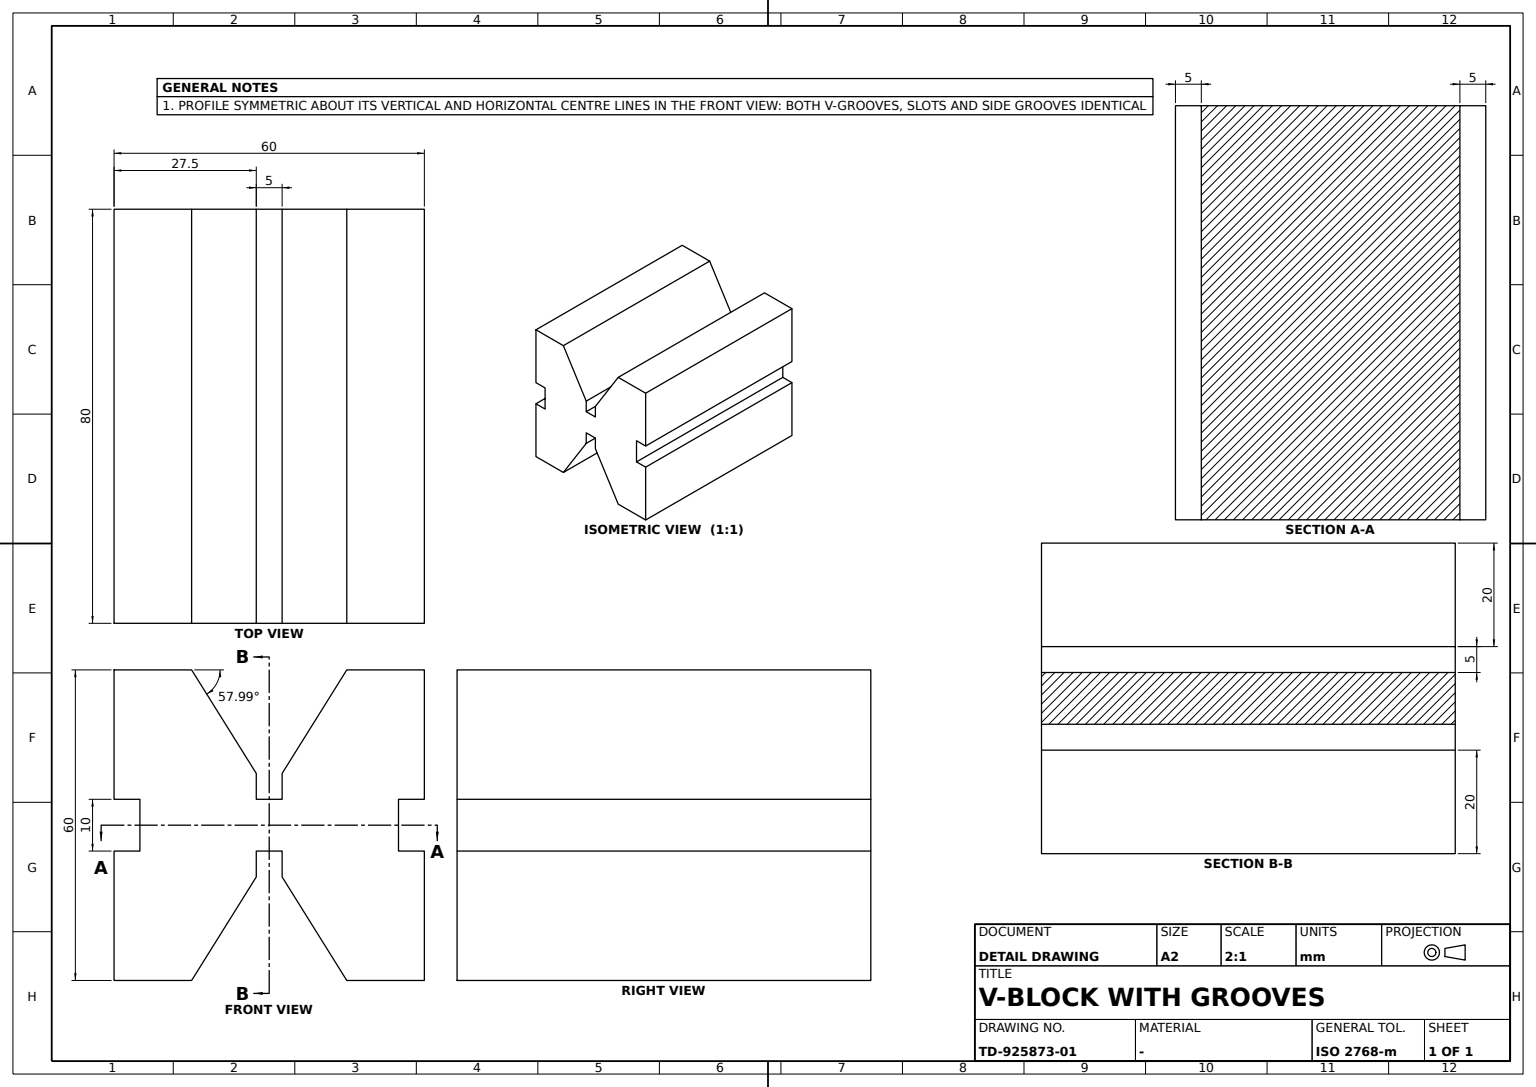
CATIA V5 part; units mm, degrees
sketch "Sketch1" plane through (0, 0, 0) normal (1, 0, 0) x (0, 1, 0)
  point P0 (15, 30)
  line L0 (15, 30) -> (30, 30)
  line L1 (30, 30) -> (30, 5)
  line L2 (30, 5) -> (25, 5)
  line L3 (25, 5) -> (25, -5)
  line L4 (25, -5) -> (30, -5)
  point P1 (30, -5)
  line L5 (30, -5) -> (30, -30)
  line L6 (30, -30) -> (15, -30)
  point P2 (15, -30)
  point P3 (0, 5)
  line L7 (0, 5) -> (2.5, 5)
  point P4 (2.5, 5)
  line L8 (2.5, 5) -> (2.5, 10)
  point P5 (2.5, 10)
  line L9 (2.5, 10) -> (15, 30)
  line L10 (0, 5) -> (0, -5)
  point P6 (0, -5)
  point P7 (15, -30)
  point P8 (2.5, -10)
  line L11 (2.5, -10) -> (15, -30)
  point P9 (2.5, -5)
  line L12 (2.5, -5) -> (2.5, -10)
  point P10 (0, -5)
  line L13 (0, -5) -> (2.5, -5)
  dimension "length L0" = 15
  dimension "length L4" = 5
  dimension "distance L2 L4" = 10
  dimension "distance L0 L6" = 60
  dimension "distance L10 P2" = 15
  dimension "length L7" = 2.5
  dimension "length L12" = 5
  dimension "length L10" = 10
  constraint horizontal L0 x-axis
  constraint horizontal L2 x-axis
  constraint horizontal L4 x-axis
  constraint horizontal L6 x-axis
  constraint horizontal L7 x-axis
  constraint vertical L1 y-axis
  constraint vertical L3 y-axis
  constraint vertical L5 y-axis
  constraint vertical L8 y-axis
  constraint vertical L10 y-axis
  constraint coincidence P1 L1
  constraint coincidence P3 y-axis
  constraint coincidence P6 P10
  constraint coincidence P2 P7
  constraint equal size L1 L5
  constraint equal size L0 L6
  constraint equal size L2 L4
  constraint symmetry L2 L4 x-axis
  constraint symmetry P0 P7 x-axis
  constraint symmetry P5 P8 x-axis
  constraint symmetry L9 L11 x-axis
  constraint symmetry P4 P9 x-axis
  constraint symmetry L8 L12 x-axis
  constraint symmetry P3 P10 x-axis
  constraint symmetry L7 L13 x-axis
extrude "Pad1" add sketch "Sketch1" along normal mid plane 80
mirror "Mirror1" about plane through (0, 0, 0) normal (0, 1, 0)
properties part number "Mechanical Stepped Clamping Block with Parallel Raised Jaws and Central Locating Slot in CATIA"
